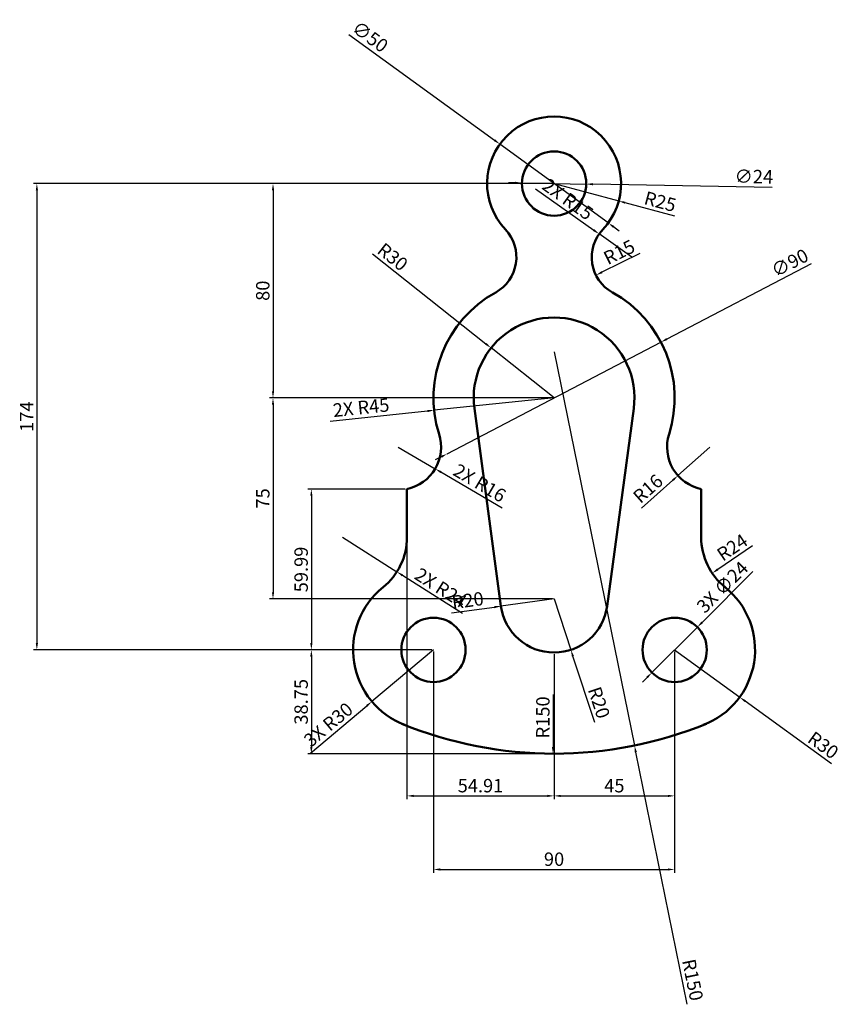
# Model space of a CAD drawing. Units: millimetres. Extents: x 2688 to 2994, y 1796 to 2164.
import ezdxf

# ---------------------------------------------------------------- set-up
doc = ezdxf.new("R2010")
doc.units = ezdxf.units.MM
doc.layers.add('M-DIMS', color=2, linetype='Continuous', lineweight=25)
doc.layers.add('M-OUTL', color=7, linetype='Continuous', lineweight=50)
doc.styles.get("Standard").update_dxf_attribs({"font": 'arial.ttf'})
doc.dimstyles.new('ISO-25', dxfattribs={"dimtxt": 5, "dimasz": 2.5, "dimexe": 1.25, "dimexo": 0.625, "dimtad": 1, "dimtxsty": 'Standard', "dimcen": 2.5, "dimadec": 0, "dimazin": 0, "dimtfac": 1, "dimtmove": 0, "dimatfit": 3, "dimfxl": 1, "dimarcsym": 0})

# ---------------------------------------------------------------- blocks, each defined once
blk = doc.blocks.new('*D1')
at = {"layer": 'Defpoints', "color": 0, "transparency": 16777216}
for p in [(2887.2, 2102.62), (2782.31, 2022.62), (2887.2, 2022.62)]:
    blk.add_point(p, dxfattribs=at)
at = {"layer": 'M-DIMS', "color": 0, "lineweight": -2, "transparency": 16777216}
for p, q in [((2886.58, 2102.62), (2781.06, 2102.62)), ((2782.31, 2100.12), (2782.31, 2025.12)), ((2886.58, 2022.62), (2781.06, 2022.62))]:
    blk.add_line(p, q, dxfattribs=at)
at = {"layer": 'M-DIMS', "color": 0, "transparency": 16777216}
for points in [[(2781.9, 2100.12), (2782.73, 2100.12), (2782.31, 2102.62)], [(2781.9, 2025.12), (2782.73, 2025.12), (2782.31, 2022.62)]]:
    blk.add_solid(points, dxfattribs=at)
at = {"layer": 'M-DIMS', "color": 0, "transparency": 16777216, "insert": (2779.14, 2062.62), "char_height": 5, "attachment_point": 5, "rotation": 90}
blk.add_mtext('80', dxfattribs=at)
blk = doc.blocks.new('*D2')
at = {"layer": 'Defpoints', "color": 0, "transparency": 16777216}
for p in [(2887.2, 2102.62), (2694.19, 1928.62), (2842.2, 1928.62)]:
    blk.add_point(p, dxfattribs=at)
at = {"layer": 'M-DIMS', "color": 0, "lineweight": -2, "transparency": 16777216}
for p, q in [((2886.58, 2102.62), (2692.94, 2102.62)), ((2694.19, 2100.12), (2694.19, 1931.12)), ((2841.58, 1928.62), (2692.94, 1928.62))]:
    blk.add_line(p, q, dxfattribs=at)
at = {"layer": 'M-DIMS', "color": 0, "transparency": 16777216}
for points in [[(2693.78, 2100.12), (2694.61, 2100.12), (2694.19, 2102.62)], [(2693.78, 1931.12), (2694.61, 1931.12), (2694.19, 1928.62)]]:
    blk.add_solid(points, dxfattribs=at)
at = {"layer": 'M-DIMS', "color": 0, "transparency": 16777216, "insert": (2691.06, 2015.62), "char_height": 5, "attachment_point": 5, "rotation": 90}
blk.add_mtext('174', dxfattribs=at)
blk = doc.blocks.new('*D3')
at = {"layer": 'Defpoints', "color": 0, "transparency": 16777216}
for p in [(2842.2, 1928.62), (2932.2, 1928.62), (2932.2, 1846.67)]:
    blk.add_point(p, dxfattribs=at)
at = {"layer": 'M-DIMS', "color": 0, "lineweight": -2, "transparency": 16777216}
for p, q in [((2842.2, 1927.99), (2842.2, 1845.42)), ((2932.2, 1927.99), (2932.2, 1845.42)), ((2844.7, 1846.67), (2929.7, 1846.67))]:
    blk.add_line(p, q, dxfattribs=at)
at = {"layer": 'M-DIMS', "color": 0, "transparency": 16777216}
for points in [[(2844.7, 1847.08), (2844.7, 1846.25), (2842.2, 1846.67)], [(2929.7, 1847.08), (2929.7, 1846.25), (2932.2, 1846.67)]]:
    blk.add_solid(points, dxfattribs=at)
at = {"layer": 'M-DIMS', "color": 0, "transparency": 16777216, "insert": (2887.2, 1849.85), "char_height": 5, "attachment_point": 5}
blk.add_mtext('90', dxfattribs=at)
blk = doc.blocks.new('*D4')
at = {"layer": 'Defpoints', "color": 0, "transparency": 16777216}
for p in [(2887.2, 2022.62), (2782.31, 1947.62), (2887.2, 1947.62)]:
    blk.add_point(p, dxfattribs=at)
at = {"layer": 'M-DIMS', "color": 0, "lineweight": -2, "transparency": 16777216}
for p, q in [((2886.58, 2022.62), (2781.06, 2022.62)), ((2782.31, 2020.12), (2782.31, 1950.12)), ((2886.58, 1947.62), (2781.06, 1947.62))]:
    blk.add_line(p, q, dxfattribs=at)
at = {"layer": 'M-DIMS', "color": 0, "transparency": 16777216}
for points in [[(2781.9, 2020.12), (2782.73, 2020.12), (2782.31, 2022.62)], [(2781.9, 1950.12), (2782.73, 1950.12), (2782.31, 1947.62)]]:
    blk.add_solid(points, dxfattribs=at)
at = {"layer": 'M-DIMS', "color": 0, "transparency": 16777216, "insert": (2779.15, 1985.12), "char_height": 5, "attachment_point": 5, "rotation": 90}
blk.add_mtext('75', dxfattribs=at)
blk = doc.blocks.new('*D5')
at = {"layer": 'Defpoints', "color": 0, "transparency": 16777216}
for p in [(2966.11, 1970.65), (2946.21, 1957.22)]:
    blk.add_point(p, dxfattribs=at)
at = {"layer": 'M-DIMS', "color": 0, "lineweight": -2, "transparency": 16777216}
blk.add_line((2961.28, 1967.39), (2948.29, 1958.62), dxfattribs=at)
at = {"layer": 'M-DIMS', "color": 0, "transparency": 16777216}
blk.add_solid([(2948.05, 1958.97), (2948.52, 1958.27), (2946.21, 1957.22)], dxfattribs=at)
at = {"layer": 'M-DIMS', "color": 0, "transparency": 16777216, "insert": (2954.07, 1966.3), "char_height": 5, "attachment_point": 5, "rotation": 34.007}
blk.add_mtext('R24', dxfattribs=at)
blk = doc.blocks.new('*D6')
at = {"layer": 'Defpoints', "color": 0, "transparency": 16777216}
for p in [(2945.38, 2004.27), (2933.44, 1993.63)]:
    blk.add_point(p, dxfattribs=at)
at = {"layer": 'M-DIMS', "color": 0, "lineweight": -2, "transparency": 16777216}
for p, q in [((2945.38, 2004.27), (2933.44, 1993.63)), ((2919.85, 1981.52), (2931.57, 1991.96))]:
    blk.add_line(p, q, dxfattribs=at)
at = {"layer": 'M-DIMS', "color": 0, "transparency": 16777216}
blk.add_solid([(2931.29, 1992.27), (2931.85, 1991.65), (2933.44, 1993.63)], dxfattribs=at)
at = {"layer": 'M-DIMS', "color": 0, "transparency": 16777216, "insert": (2922.66, 1988.28), "char_height": 5, "attachment_point": 5, "rotation": 41.7075}
blk.add_mtext('R16', dxfattribs=at)
blk = doc.blocks.new('*D7')
at = {"layer": 'Defpoints', "color": 0, "transparency": 16777216}
for p in [(2916.25, 2075.12), (2902.84, 2068.41)]:
    blk.add_point(p, dxfattribs=at)
at = {"layer": 'M-DIMS', "color": 0, "lineweight": -2, "transparency": 16777216}
blk.add_line((2919.15, 2076.56), (2905.07, 2069.52), dxfattribs=at)
at = {"layer": 'M-DIMS', "color": 0, "transparency": 16777216}
blk.add_solid([(2904.89, 2069.9), (2905.26, 2069.15), (2902.84, 2068.41)], dxfattribs=at)
at = {"layer": 'M-DIMS', "color": 0, "transparency": 16777216, "insert": (2911.8, 2076.45), "char_height": 5, "attachment_point": 5, "rotation": 26.5756}
blk.add_mtext('R15', dxfattribs=at)
blk = doc.blocks.new('*D8')
at = {"layer": 'Defpoints', "color": 0, "transparency": 16777216}
for p in [(2887.2, 1947.62), (2893.46, 1928.62)]:
    blk.add_point(p, dxfattribs=at)
at = {"layer": 'M-DIMS', "color": 0, "lineweight": -2, "transparency": 16777216}
for p, q in [((2887.2, 1947.62), (2893.46, 1928.62)), ((2902.4, 1901.47), (2894.24, 1926.25))]:
    blk.add_line(p, q, dxfattribs=at)
at = {"layer": 'M-DIMS', "color": 0, "transparency": 16777216}
blk.add_solid([(2894.64, 1926.38), (2893.85, 1926.12), (2893.46, 1928.62)], dxfattribs=at)
at = {"layer": 'M-DIMS', "color": 0, "transparency": 16777216, "insert": (2903.36, 1908.73), "char_height": 5, "attachment_point": 5, "rotation": 288.2266}
blk.add_mtext('R20', dxfattribs=at)
blk = doc.blocks.new('*D9')
at = {"layer": 'Defpoints', "color": 0, "transparency": 16777216}
for p in [(2932.2, 1928.62), (2956.47, 1910.98)]:
    blk.add_point(p, dxfattribs=at)
at = {"layer": 'M-DIMS', "color": 0, "lineweight": -2, "transparency": 16777216}
for p, q in [((2932.2, 1928.62), (2956.47, 1910.98)), ((2990.74, 1886.07), (2958.49, 1909.51))]:
    blk.add_line(p, q, dxfattribs=at)
at = {"layer": 'M-DIMS', "color": 0, "transparency": 16777216}
blk.add_solid([(2958.74, 1909.85), (2958.25, 1909.17), (2956.47, 1910.98)], dxfattribs=at)
at = {"layer": 'M-DIMS', "color": 0, "transparency": 16777216, "insert": (2987.28, 1892.51), "char_height": 5, "attachment_point": 5, "rotation": 323.9884}
blk.add_mtext('R30', dxfattribs=at)
blk = doc.blocks.new('*D10')
at = {"layer": 'Defpoints', "color": 0, "transparency": 16777216}
for p in [(2875.21, 2102.83), (2899.2, 2102.4)]:
    blk.add_point(p, dxfattribs=at)
at = {"layer": 'M-DIMS', "color": 0, "lineweight": -2, "transparency": 16777216}
for p, q in [((2872.71, 2102.88), (2870.21, 2102.92)), ((2875.21, 2102.83), (2899.2, 2102.4)), ((2968.61, 2101.14), (2901.7, 2102.35))]:
    blk.add_line(p, q, dxfattribs=at)
at = {"layer": 'M-DIMS', "color": 0, "transparency": 16777216}
for points in [[(2872.71, 2103.3), (2872.7, 2102.46), (2875.21, 2102.83)], [(2901.71, 2102.77), (2901.69, 2101.94), (2899.2, 2102.4)]]:
    blk.add_solid(points, dxfattribs=at)
at = {"layer": 'M-DIMS', "color": 0, "transparency": 16777216, "insert": (2961.76, 2104.58), "char_height": 5, "attachment_point": 5, "rotation": 358.9623}
blk.add_mtext('∅24', dxfattribs=at)
blk = doc.blocks.new('*D11')
at = {"layer": 'Defpoints', "color": 0, "transparency": 16777216}
for p in [(2866.98, 2117.31), (2907.43, 2087.92)]:
    blk.add_point(p, dxfattribs=at)
at = {"layer": 'M-DIMS', "color": 0, "lineweight": -2, "transparency": 16777216}
for p, q in [((2810.63, 2158.25), (2864.96, 2118.78)), ((2907.43, 2087.92), (2866.98, 2117.31)), ((2909.45, 2086.45), (2911.48, 2084.98))]:
    blk.add_line(p, q, dxfattribs=at)
at = {"layer": 'M-DIMS', "color": 0, "transparency": 16777216}
for points in [[(2865.2, 2119.12), (2864.71, 2118.44), (2866.98, 2117.31)], [(2909.7, 2086.79), (2909.21, 2086.12), (2907.43, 2087.92)]]:
    blk.add_solid(points, dxfattribs=at)
at = {"layer": 'M-DIMS', "color": 0, "transparency": 16777216, "insert": (2818.18, 2156.87), "char_height": 5, "attachment_point": 5, "rotation": 324.0006}
blk.add_mtext('∅50', dxfattribs=at)
blk = doc.blocks.new('*D12')
at = {"layer": 'Defpoints', "color": 0, "transparency": 16777216}
for p in [(2927.1, 2043.44), (2847.31, 2001.79)]:
    blk.add_point(p, dxfattribs=at)
at = {"layer": 'M-DIMS', "color": 0, "lineweight": -2, "transparency": 16777216}
for p, q in [((2983.13, 2072.7), (2929.31, 2044.6)), ((2847.31, 2001.79), (2927.1, 2043.44)), ((2845.1, 2000.63), (2842.88, 1999.48))]:
    blk.add_line(p, q, dxfattribs=at)
at = {"layer": 'M-DIMS', "color": 0, "transparency": 16777216}
for points in [[(2929.12, 2044.97), (2929.5, 2044.23), (2927.1, 2043.44)], [(2844.9, 2001), (2845.29, 2000.27), (2847.31, 2001.79)]]:
    blk.add_solid(points, dxfattribs=at)
at = {"layer": 'M-DIMS', "color": 0, "transparency": 16777216, "insert": (2975.47, 2072.44), "char_height": 5, "attachment_point": 5, "rotation": 27.5666}
blk.add_mtext('∅90', dxfattribs=at)
blk = doc.blocks.new('*D13')
at = {"layer": 'Defpoints', "color": 0, "transparency": 16777216}
for p in [(2887.2, 2039.87), (2886.8, 1889.87)]:
    blk.add_point(p, dxfattribs=at)
at = {"layer": 'M-DIMS', "color": 0, "lineweight": -2, "transparency": 16777216}
blk.add_line((2886.86, 1911.93), (2886.81, 1892.37), dxfattribs=at)
at = {"layer": 'M-DIMS', "color": 0, "transparency": 16777216}
blk.add_solid([(2886.39, 1892.37), (2887.22, 1892.36), (2886.8, 1889.87)], dxfattribs=at)
at = {"layer": 'M-DIMS', "color": 0, "transparency": 16777216, "insert": (2883.66, 1903.41), "char_height": 5, "attachment_point": 5, "rotation": 89.8457}
blk.add_mtext('R150', dxfattribs=at)
blk = doc.blocks.new('*D14')
at = {"layer": 'Defpoints', "color": 0, "transparency": 16777216}
for p in [(2863.69, 2041.25), (2887.2, 2022.62)]:
    blk.add_point(p, dxfattribs=at)
at = {"layer": 'M-DIMS', "color": 0, "lineweight": -2, "transparency": 16777216}
for p, q in [((2819.43, 2076.33), (2861.73, 2042.8)), ((2887.2, 2022.62), (2863.69, 2041.25))]:
    blk.add_line(p, q, dxfattribs=at)
at = {"layer": 'M-DIMS', "color": 0, "transparency": 16777216}
blk.add_solid([(2861.99, 2043.13), (2861.47, 2042.48), (2863.69, 2041.25)], dxfattribs=at)
at = {"layer": 'M-DIMS', "color": 0, "transparency": 16777216, "insert": (2826.57, 2074.72), "char_height": 5, "attachment_point": 5, "rotation": 321.6047}
blk.add_mtext('R30', dxfattribs=at)
blk = doc.blocks.new('HOLE-D24')
blk.add_circle((12, 12), 12)
blk = doc.blocks.new('*D16')
at = {"layer": 'Defpoints', "color": 0, "transparency": 16777216}
for p in [(2842.2, 1928.62), (2796.62, 1889.87), (2887.2, 1889.87)]:
    blk.add_point(p, dxfattribs=at)
at = {"layer": 'M-DIMS', "color": 0, "lineweight": -2, "transparency": 16777216}
for p, q in [((2841.58, 1928.62), (2795.37, 1928.62)), ((2796.62, 1926.12), (2796.62, 1892.37)), ((2886.58, 1889.87), (2795.37, 1889.87))]:
    blk.add_line(p, q, dxfattribs=at)
at = {"layer": 'M-DIMS', "color": 0, "transparency": 16777216}
for points in [[(2796.21, 1926.12), (2797.04, 1926.12), (2796.62, 1928.62)], [(2796.21, 1892.37), (2797.04, 1892.37), (2796.62, 1889.87)]]:
    blk.add_solid(points, dxfattribs=at)
at = {"layer": 'M-DIMS', "color": 0, "transparency": 16777216, "insert": (2793.45, 1909.24), "char_height": 5, "attachment_point": 5, "rotation": 90}
blk.add_mtext('38.75', dxfattribs=at)
blk = doc.blocks.new('*D17')
at = {"layer": 'Defpoints', "color": 0, "transparency": 16777216}
for p in [(2832.3, 1988.61), (2796.62, 1928.62), (2842.2, 1928.62)]:
    blk.add_point(p, dxfattribs=at)
at = {"layer": 'M-DIMS', "color": 0, "lineweight": -2, "transparency": 16777216}
for p, q in [((2831.67, 1988.61), (2795.37, 1988.61)), ((2796.62, 1986.11), (2796.62, 1931.12)), ((2841.58, 1928.62), (2795.37, 1928.62))]:
    blk.add_line(p, q, dxfattribs=at)
at = {"layer": 'M-DIMS', "color": 0, "transparency": 16777216}
for points in [[(2796.21, 1986.11), (2797.04, 1986.11), (2796.62, 1988.61)], [(2796.21, 1931.12), (2797.04, 1931.12), (2796.62, 1928.62)]]:
    blk.add_solid(points, dxfattribs=at)
at = {"layer": 'M-DIMS', "color": 0, "transparency": 16777216, "insert": (2793.45, 1958.61), "char_height": 5, "attachment_point": 5, "rotation": 90}
blk.add_mtext('59.99', dxfattribs=at)
blk = doc.blocks.new('*D18')
at = {"layer": 'Defpoints', "color": 0, "transparency": 16777216}
for p in [(2832.3, 1970.65), (2887.2, 1927.62), (2887.2, 1874.12)]:
    blk.add_point(p, dxfattribs=at)
at = {"layer": 'M-DIMS', "color": 0, "lineweight": -2, "transparency": 16777216}
for p, q in [((2832.3, 1970.02), (2832.3, 1872.87)), ((2887.2, 1926.99), (2887.2, 1872.87)), ((2834.8, 1874.12), (2884.7, 1874.12))]:
    blk.add_line(p, q, dxfattribs=at)
at = {"layer": 'M-DIMS', "color": 0, "transparency": 16777216}
for points in [[(2834.8, 1874.53), (2834.8, 1873.7), (2832.3, 1874.12)], [(2884.7, 1874.53), (2884.7, 1873.7), (2887.2, 1874.12)]]:
    blk.add_solid(points, dxfattribs=at)
at = {"layer": 'M-DIMS', "color": 0, "transparency": 16777216, "insert": (2859.75, 1877.29), "char_height": 5, "attachment_point": 5}
blk.add_mtext('54.91', dxfattribs=at)
blk = doc.blocks.new('*D19')
at = {"layer": 'Defpoints', "color": 0, "transparency": 16777216}
for p in [(2887.2, 1927.62), (2932.2, 1928.62), (2932.2, 1874.12)]:
    blk.add_point(p, dxfattribs=at)
at = {"layer": 'M-DIMS', "color": 0, "lineweight": -2, "transparency": 16777216}
for p, q in [((2887.2, 1926.99), (2887.2, 1872.87)), ((2932.2, 1927.99), (2932.2, 1872.87)), ((2889.7, 1874.12), (2929.7, 1874.12))]:
    blk.add_line(p, q, dxfattribs=at)
at = {"layer": 'M-DIMS', "color": 0, "transparency": 16777216}
for points in [[(2889.7, 1874.53), (2889.7, 1873.7), (2887.2, 1874.12)], [(2929.7, 1874.53), (2929.7, 1873.7), (2932.2, 1874.12)]]:
    blk.add_solid(points, dxfattribs=at)
at = {"layer": 'M-DIMS', "color": 0, "transparency": 16777216, "insert": (2909.7, 1877.28), "char_height": 5, "attachment_point": 5}
blk.add_mtext('45', dxfattribs=at)
blk = doc.blocks.new('*D20')
at = {"layer": 'Defpoints', "color": 0, "transparency": 16777216}
for p in [(2940.69, 1937.1), (2923.72, 1920.13)]:
    blk.add_point(p, dxfattribs=at)
at = {"layer": 'M-DIMS', "color": 0, "lineweight": -2, "transparency": 16777216}
for p, q in [((2961.42, 1957.82), (2942.46, 1938.87)), ((2923.72, 1920.13), (2940.69, 1937.1)), ((2921.95, 1918.36), (2920.18, 1916.6))]:
    blk.add_line(p, q, dxfattribs=at)
at = {"layer": 'M-DIMS', "color": 0, "transparency": 16777216}
for points in [[(2942.16, 1939.16), (2942.75, 1938.57), (2940.69, 1937.1)], [(2921.66, 1918.66), (2922.24, 1918.07), (2923.72, 1920.13)]]:
    blk.add_solid(points, dxfattribs=at)
at = {"layer": 'M-DIMS', "color": 0, "transparency": 16777216, "insert": (2950.48, 1951.57), "char_height": 5, "attachment_point": 5, "rotation": 44.9925}
blk.add_mtext('3X ∅24', dxfattribs=at)
blk = doc.blocks.new('*D21')
at = {"layer": 'Defpoints', "color": 0, "transparency": 16777216}
for p in [(2887.2, 2102.62), (2911.34, 2096.1)]:
    blk.add_point(p, dxfattribs=at)
at = {"layer": 'M-DIMS', "color": 0, "lineweight": -2, "transparency": 16777216}
for p, q in [((2887.2, 2102.62), (2911.34, 2096.1)), ((2932.21, 2090.46), (2913.75, 2095.45))]:
    blk.add_line(p, q, dxfattribs=at)
at = {"layer": 'M-DIMS', "color": 0, "transparency": 16777216}
blk.add_solid([(2913.86, 2095.85), (2913.65, 2095.05), (2911.34, 2096.1)], dxfattribs=at)
at = {"layer": 'M-DIMS', "color": 0, "transparency": 16777216, "insert": (2926.65, 2095.26), "char_height": 5, "attachment_point": 5, "rotation": 344.8903}
blk.add_mtext('R25', dxfattribs=at)
blk = doc.blocks.new('*D22')
at = {"layer": 'Defpoints', "color": 0, "transparency": 16777216}
for p in [(2904.02, 2083.8), (2916.25, 2075.12)]:
    blk.add_point(p, dxfattribs=at)
at = {"layer": 'M-DIMS', "color": 0, "lineweight": -2, "transparency": 16777216}
for p, q in [((2880.32, 2100.62), (2901.98, 2085.25)), ((2916.25, 2075.12), (2904.02, 2083.8))]:
    blk.add_line(p, q, dxfattribs=at)
at = {"layer": 'M-DIMS', "color": 0, "transparency": 16777216}
blk.add_solid([(2902.22, 2085.59), (2901.74, 2084.91), (2904.02, 2083.8)], dxfattribs=at)
at = {"layer": 'M-DIMS', "color": 0, "transparency": 16777216, "insert": (2891.97, 2096.25), "char_height": 5, "attachment_point": 5, "rotation": 324.6282}
blk.add_mtext('2X R15', dxfattribs=at)
blk = doc.blocks.new('*D23')
at = {"layer": 'Defpoints', "color": 0, "transparency": 16777216}
for p in [(2887.2, 2022.62), (2842.44, 2018)]:
    blk.add_point(p, dxfattribs=at)
at = {"layer": 'M-DIMS', "color": 0, "lineweight": -2, "transparency": 16777216}
for p, q in [((2887.2, 2022.62), (2842.44, 2018)), ((2803.62, 2014), (2839.96, 2017.74))]:
    blk.add_line(p, q, dxfattribs=at)
at = {"layer": 'M-DIMS', "color": 0, "transparency": 16777216}
blk.add_solid([(2839.91, 2018.16), (2840, 2017.33), (2842.44, 2018)], dxfattribs=at)
at = {"layer": 'M-DIMS', "color": 0, "transparency": 16777216, "insert": (2815.26, 2018.39), "char_height": 5, "attachment_point": 5, "rotation": 5.8882}
blk.add_mtext('2X R45', dxfattribs=at)
blk = doc.blocks.new('*D24')
at = {"layer": 'Defpoints', "color": 0, "transparency": 16777216}
for p in [(2829.03, 2004.27), (2842.84, 1996.19)]:
    blk.add_point(p, dxfattribs=at)
at = {"layer": 'M-DIMS', "color": 0, "lineweight": -2, "transparency": 16777216}
for p, q in [((2829.03, 2004.27), (2842.84, 1996.19)), ((2867.88, 1981.52), (2844.99, 1994.92))]:
    blk.add_line(p, q, dxfattribs=at)
at = {"layer": 'M-DIMS', "color": 0, "transparency": 16777216}
blk.add_solid([(2845.2, 1995.28), (2844.78, 1994.56), (2842.84, 1996.19)], dxfattribs=at)
at = {"layer": 'M-DIMS', "color": 0, "transparency": 16777216, "insert": (2859.12, 1990.33), "char_height": 5, "attachment_point": 5, "rotation": 329.6473}
blk.add_mtext('2X R16', dxfattribs=at)
blk = doc.blocks.new('*D25')
at = {"layer": 'Defpoints', "color": 0, "transparency": 16777216}
for p in [(2808.3, 1970.65), (2828.54, 1957.74)]:
    blk.add_point(p, dxfattribs=at)
at = {"layer": 'M-DIMS', "color": 0, "lineweight": -2, "transparency": 16777216}
for p, q in [((2808.3, 1970.65), (2828.54, 1957.74)), ((2853, 1942.15), (2830.64, 1956.4))]:
    blk.add_line(p, q, dxfattribs=at)
at = {"layer": 'M-DIMS', "color": 0, "transparency": 16777216}
blk.add_solid([(2830.87, 1956.75), (2830.42, 1956.05), (2828.54, 1957.74)], dxfattribs=at)
at = {"layer": 'M-DIMS', "color": 0, "transparency": 16777216, "insert": (2844.56, 1951.25), "char_height": 5, "attachment_point": 5, "rotation": 327.485}
blk.add_mtext('2X R24', dxfattribs=at)
blk = doc.blocks.new('*D26')
at = {"layer": 'Defpoints', "color": 0, "transparency": 16777216}
for p in [(2842.2, 1928.62), (2819.22, 1909.34)]:
    blk.add_point(p, dxfattribs=at)
at = {"layer": 'M-DIMS', "color": 0, "lineweight": -2, "transparency": 16777216}
for p, q in [((2842.2, 1928.62), (2819.22, 1909.34)), ((2796.26, 1890.09), (2817.3, 1907.73))]:
    blk.add_line(p, q, dxfattribs=at)
at = {"layer": 'M-DIMS', "color": 0, "transparency": 16777216}
blk.add_solid([(2817.04, 1908.05), (2817.57, 1907.41), (2819.22, 1909.34)], dxfattribs=at)
at = {"layer": 'M-DIMS', "color": 0, "transparency": 16777216, "insert": (2803.38, 1900.21), "char_height": 5, "attachment_point": 5, "rotation": 39.986}
blk.add_mtext('3X R30', dxfattribs=at)
blk = doc.blocks.new('*D27')
at = {"layer": 'Defpoints', "color": 0, "transparency": 16777216}
for p in [(2887.2, 1947.62), (2867.39, 1944.9)]:
    blk.add_point(p, dxfattribs=at)
at = {"layer": 'M-DIMS', "color": 0, "lineweight": -2, "transparency": 16777216}
for p, q in [((2887.2, 1947.62), (2867.39, 1944.9)), ((2848.97, 1942.37), (2864.91, 1944.56))]:
    blk.add_line(p, q, dxfattribs=at)
at = {"layer": 'M-DIMS', "color": 0, "transparency": 16777216}
blk.add_solid([(2864.86, 1944.97), (2864.97, 1944.15), (2867.39, 1944.9)], dxfattribs=at)
at = {"layer": 'M-DIMS', "color": 0, "transparency": 16777216, "insert": (2855.07, 1946.42), "char_height": 5, "attachment_point": 5, "rotation": 7.8107}
blk.add_mtext('R20', dxfattribs=at)
blk = doc.blocks.new('*D28')
at = {"layer": 'Defpoints', "color": 0, "transparency": 16777216}
for p in [(2887.2, 2039.87), (2917.2, 1892.9)]:
    blk.add_point(p, dxfattribs=at)
at = {"layer": 'M-DIMS', "color": 0, "lineweight": -2, "transparency": 16777216}
for p, q in [((2887.2, 2039.87), (2917.2, 1892.9)), ((2936.91, 1796.35), (2917.7, 1890.45))]:
    blk.add_line(p, q, dxfattribs=at)
at = {"layer": 'M-DIMS', "color": 0, "transparency": 16777216}
blk.add_solid([(2918.11, 1890.53), (2917.3, 1890.36), (2917.2, 1892.9)], dxfattribs=at)
at = {"layer": 'M-DIMS', "color": 0, "transparency": 16777216, "insert": (2938.32, 1805.35), "char_height": 5, "attachment_point": 5, "rotation": 281.5371}
blk.add_mtext('R150', dxfattribs=at)

msp = doc.modelspace()

# ---------------------------------------------------------------- linework, layer by layer
at = {"layer": 'M-OUTL'}
for p, q in [((2857.472, 2018.617), (2867.383, 1944.95)), ((2916.937, 2018.617), (2907.026, 1944.95)), ((2832.299, 1988.61), (2832.299, 1970.645)), ((2942.11, 1988.61), (2942.11, 1970.645))]:
    msp.add_line(p, q, dxfattribs=at)
for centre, radius, start, end in [((2887.204, 2102.617), 25, 316.56746, 223.43254), ((2858.157, 2075.117), 15, 298.95502, 43.43254), ((2916.252, 2075.117), 15, 136.56746, 241.04498), ((2887.204, 2022.617), 45, 118.95502, 197.50148), ((2887.204, 2022.617), 45, 342.49852, 61.04498), ((2887.204, 2022.617), 30, 352.33774, 187.66226), ((2829.028, 2004.272), 16, 281.79476, 17.50148), ((2945.381, 2004.272), 16, 162.49852, 258.20524), ((2808.299, 1970.645), 24, 308.89421, 360), ((2966.11, 1970.645), 24, 180, 231.10579), ((2842.204, 1928.617), 30, 128.89421, 249.18984), ((2932.204, 1928.617), 30, 290.81016, 51.10579), ((2887.204, 1947.617), 20, 187.66226, 352.33774), ((2887.204, 2039.865), 150, 247.73412, 292.26588)]:
    msp.add_arc(centre, radius, start, end, dxfattribs=at)

# ---------------------------------------------------------------- block references
for p in [(2875.204, 2090.617), (2830.204, 1916.617), (2920.204, 1916.617)]:
    msp.add_blockref('HOLE-D24', p, dxfattribs=at)

# ---------------------------------------------------------------- dimensions: what is measured, and where the dimension line sits
at = {"layer": 'M-DIMS'}
for p1, p2, picture, middle in [((2907.43, 2087.922), (2866.979, 2117.311), '*D11', (2816.231, 2154.181)), ((2875.206, 2102.834), (2899.202, 2102.399), '*D10', (2961.697, 2101.267)), ((2847.313, 2001.792), (2927.096, 2043.442), '*D12', (2977.002, 2069.495))]:
    dim = msp.add_diameter_dim_2p(p1=p1, p2=p2, dimstyle='ISO-25', override={"dimclrd": 0, "dimclre": 0, "dimclrt": 0}, dxfattribs=at)
    dim.commit()
    dim.dimension.update_dxf_attribs({"geometry": picture, "text_midpoint": middle, "dimtype": 163})
for center, mpoint, picture, middle in [((2916.252, 2075.117), (2904.021, 2083.8), '*D22', (2891.972, 2096.251)), ((2829.028, 2004.272), (2842.835, 1996.187), '*D24', (2859.121, 1990.333)), ((2808.299, 1970.645), (2828.537, 1957.745), '*D25', (2844.561, 1951.251))]:
    dim = msp.add_radius_dim(center=center, mpoint=mpoint, text='2X <>', dimstyle='ISO-25', override={"dimdec": 0, "dimlfac": 1, "dimrnd": 0, "dimzin": 0, "dimdsep": 46, "dimlunit": 2}, dxfattribs=at)
    dim.commit()
    dim.dimension.update_dxf_attribs({"geometry": picture, "text_midpoint": middle})
for base, p1, p2, override, picture, middle in [((2694.192, 1928.617), (2887.204, 2102.617), (2842.204, 1928.617), {"dimclrd": 0, "dimclre": 0, "dimclrt": 0}, '*D2', (2691.057, 2015.617)), ((2782.315, 2022.617), (2887.204, 2102.617), (2887.204, 2022.617), {"dimclrd": 0, "dimclre": 0, "dimclrt": 0}, '*D1', (2779.137, 2062.617)), ((2782.315, 1947.617), (2887.204, 2022.617), (2887.204, 1947.617), {"dimclrd": 0, "dimclre": 0, "dimclrt": 0}, '*D4', (2779.147, 1985.117)), ((2796.625, 1928.617), (2832.299, 1988.61), (2842.204, 1928.617), {"dimdec": 2, "dimlfac": 1, "dimrnd": 0, "dimzin": 0, "dimdsep": 46, "dimlunit": 2}, '*D17', (2793.447, 1958.613)), ((2796.625, 1889.865), (2842.204, 1928.617), (2887.204, 1889.865), {"dimdec": 2, "dimlfac": 1, "dimrnd": 0, "dimzin": 0, "dimdsep": 46, "dimlunit": 2}, '*D16', (2793.445, 1909.241))]:
    dim = msp.add_linear_dim(base=base, p1=p1, p2=p2, angle=90, dimstyle='ISO-25', override=override, dxfattribs=at)
    dim.commit()
    dim.dimension.update_dxf_attribs({"geometry": picture, "text_midpoint": middle})
for center, mpoint, override, picture, middle in [((2887.204, 2102.617), (2911.34, 2096.1), {"dimdec": 0, "dimlfac": 1, "dimrnd": 0, "dimzin": 0, "dimdsep": 46, "dimlunit": 2}, '*D21', (2925.822, 2092.19)), ((2887.204, 2022.617), (2863.692, 2041.249), {"dimclrd": 0, "dimclre": 0, "dimclrt": 0}, '*D14', (2824.594, 2072.233)), ((2916.252, 2075.117), (2902.837, 2068.406), {"dimclrd": 0, "dimclre": 0, "dimclrt": 0}, '*D7', (2913.227, 2073.603)), ((2887.204, 2039.865), (2886.801, 1889.866), {"dimclrd": 0, "dimclre": 0, "dimclrt": 0}, '*D13', (2886.837, 1903.398)), ((2887.204, 2039.865), (2917.205, 1892.896), {"dimdec": 0, "dimlfac": 1, "dimrnd": 0, "dimzin": 0, "dimdsep": 46, "dimlunit": 2}, '*D28', (2935.205, 1804.715)), ((2966.11, 1970.645), (2946.215, 1957.222), {"dimclrd": 0, "dimclre": 0, "dimclrt": 0}, '*D5', (2955.821, 1963.704)), ((2887.204, 1947.617), (2867.39, 1944.899), {"dimdec": 0, "dimlfac": 1, "dimrnd": 0, "dimzin": 0, "dimdsep": 46, "dimlunit": 2}, '*D27', (2855.501, 1943.268)), ((2887.204, 1947.617), (2893.46, 1928.62), {"dimclrd": 0, "dimclre": 0, "dimclrt": 0}, '*D8', (2900.338, 1907.735)), ((2932.204, 1928.617), (2956.471, 1910.978), {"dimclrd": 0, "dimclre": 0, "dimclrt": 0}, '*D9', (2985.412, 1889.943))]:
    dim = msp.add_radius_dim(center=center, mpoint=mpoint, dimstyle='ISO-25', override=override, dxfattribs=at)
    dim.commit()
    dim.dimension.update_dxf_attribs({"geometry": picture, "text_midpoint": middle, "dimtype": 164})
for center, mpoint, text, picture, middle in [((2887.204, 2022.617), (2842.442, 2018), '2X <>', '*D23', (2815.584, 2015.23)), ((2842.204, 1928.617), (2819.218, 1909.339), '3X <>', '*D26', (2805.427, 1897.772))]:
    dim = msp.add_radius_dim(center=center, mpoint=mpoint, text=text, dimstyle='ISO-25', override={"dimdec": 0, "dimlfac": 1, "dimrnd": 0, "dimzin": 0, "dimdsep": 46, "dimlunit": 2}, dxfattribs=at)
    dim.commit()
    dim.dimension.update_dxf_attribs({"geometry": picture, "text_midpoint": middle, "dimtype": 164})
dim = msp.add_radius_dim(center=(2945.381, 2004.272), mpoint=(2933.436, 1993.627), dimstyle='ISO-25', override={"dimclrd": 0, "dimclre": 0, "dimclrt": 0}, dxfattribs=at)
dim.commit()
dim.dimension.update_dxf_attribs({"geometry": '*D6', "text_midpoint": (2922.664, 1988.283)})
for base, p1, p2, override, picture, middle in [((2887.2044, 1874.1154), (2832.2987, 1970.6452), (2887.2044, 1927.6167), {"dimdec": 2, "dimlfac": 1, "dimrnd": 0, "dimzin": 0, "dimdsep": 46, "dimlunit": 2}, '*D18', (2859.7516, 1877.2933)), ((2932.204, 1846.668), (2842.204, 1928.617), (2932.204, 1928.617), {"dimclrd": 0, "dimclre": 0, "dimclrt": 0}, '*D3', (2887.204, 1849.845)), ((2932.204, 1874.115), (2887.204, 1927.617), (2932.204, 1928.617), {"dimdec": 0, "dimlfac": 1, "dimrnd": 0, "dimzin": 0, "dimdsep": 46, "dimlunit": 2}, '*D19', (2909.704, 1877.283))]:
    dim = msp.add_linear_dim(base=base, p1=p1, p2=p2, dimstyle='ISO-25', override=override, dxfattribs=at)
    dim.commit()
    dim.dimension.update_dxf_attribs({"geometry": picture, "text_midpoint": middle})
dim = msp.add_diameter_dim_2p(p1=(2923.718, 1920.132), p2=(2940.691, 1937.101), text='3X <>', dimstyle='ISO-25', override={"dimdec": 0, "dimlfac": 1, "dimrnd": 0, "dimzin": 0, "dimdsep": 46, "dimlunit": 2}, dxfattribs=at)
dim.commit()
dim.dimension.update_dxf_attribs({"geometry": '*D20', "text_midpoint": (2952.821, 1949.228)})

doc.saveas('drawing.dxf')
